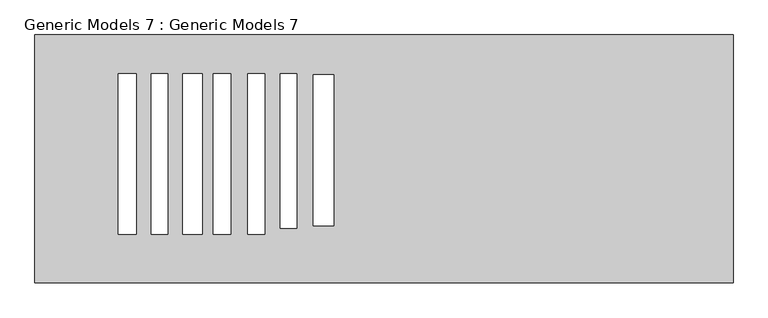
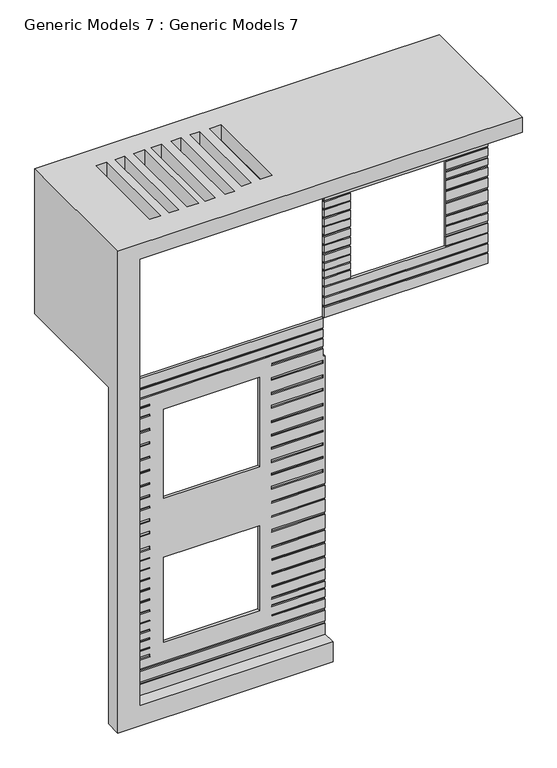
"""IFC4 building model written with IfcOpenShell, lengths in millimetres: proxy geometry, Generic Models 7 : Generic Models 7."""

from ifc_helpers import new_model, si_unit, origin, place, context, project, spatial, faceted_brep, source, transform, mapped, element, save


def generic_models_7_generic_models_7_94141b15(model_context):
    return source(origin(), model_context, "Body", "Brep", [
        faceted_brep([(-19866.491855, -13904.9538163, 3044.3262356), (-19256.891855, -13904.9538163, 3044.3262356), (-19256.891855, -13904.9538163, 3048.6001668), (-17428.091855, -13904.9538163, 3048.6001668), (-17428.091855, -13904.9538163, 3047.830136), (-16170.791855, -13904.9538163, 3047.830136), (-16170.791855, -13904.9538163, 3267.9963637), (-19866.491855, -13904.9538163, 3267.9963637), (-16208.891855, -13904.9538163, 9448.8), (-19866.491855, -13904.9538163, 9448.8), (-19866.491855, -13904.9538163, 9255.7850961), (-16208.891855, -13904.9538163, 9255.7850961), (-16170.791855, -13904.9538163, 8676.8631794), (-16208.891855, -13904.9538163, 8676.8631794), (-16208.891855, -13904.9538163, 8832.7952088), (-17199.491855, -13904.9538163, 8832.7952088), (-17199.491855, -13904.9538163, 8880.0631794), (-16208.891855, -13904.9538163, 8880.0631794), (-16208.891855, -13904.9538163, 9029.746389), (-19866.491855, -13904.9538163, 9029.746389), (-19866.491855, -13904.9538163, 8880.0631794), (-19518.8909009, -13904.9538163, 8880.0631794), (-19518.8909009, -13904.9538163, 8832.7952088), (-19866.491855, -13904.9538163, 8832.7952088), (-19866.491855, -13904.9538163, 8676.8631794), (-19518.8909009, -13904.9538163, 8676.8631794), (-19518.8909009, -13904.9538163, 8634.1909778), (-19866.491855, -13904.9538163, 8634.1909778), (-19866.491855, -13904.9538163, 8392.6341349), (-19518.8909009, -13904.9538163, 8392.6341349), (-19518.8909009, -13904.9538163, 8341.0204513), (-19866.491855, -13904.9538163, 8341.0204513), (-19866.491855, -13904.9538163, 8123.1111078), (-19518.8909009, -13904.9538163, 8123.1111078), (-19518.8909009, -13904.9538163, 8063.5568574), (-19866.491855, -13904.9538163, 8063.5568574), (-19866.491855, -13904.9538163, 7829.3101393), (-19518.8909009, -13904.9538163, 7829.3101393), (-19518.8909009, -13904.9538163, 7789.6073057), (-19866.491855, -13904.9538163, 7789.6073057), (-19866.491855, -13904.9538163, 7560.8382052), (-19518.8909009, -13904.9538163, 7560.8382052), (-19518.8909009, -13904.9538163, 7519.6280374), (-19866.491855, -13904.9538163, 7519.6280374), (-19866.491855, -13904.9538163, 7292.9915007), (-19518.8909009, -13904.9538163, 7292.9915007), (-19518.8909009, -13904.9538163, 7245.6784857), (-19866.491855, -13904.9538163, 7245.6784857), (-19866.491855, -13904.9538163, 7047.1643178), (-19518.8909009, -13904.9538163, 7047.1643178), (-19518.8909009, -13904.9538163, 6995.5506342), (-19866.491855, -13904.9538163, 6995.5506342), (-19866.491855, -13904.9538163, 6812.9175997), (-19518.8909009, -13904.9538163, 6812.9175997), (-19518.8909009, -13904.9538163, 6777.1850495), (-19866.491855, -13904.9538163, 6777.1850495), (-19866.491855, -13904.9538163, 6565.3056423), (-19518.8909009, -13904.9538163, 6565.3056423), (-19518.8909009, -13904.9538163, 6498.8842905), (-19866.491855, -13904.9538163, 6498.8842905), (-19866.491855, -13904.9538163, 6314.0836024), (-19518.8909009, -13904.9538163, 6314.0836024), (-19518.8909009, -13904.9538163, 6245.8245058), (-19866.491855, -13904.9538163, 6245.8245058), (-19866.491855, -13904.9538163, 6004.2923177), (-19518.8909009, -13904.9538163, 6004.2923177), (-19518.8909009, -13904.9538163, 5941.2839209), (-19866.491855, -13904.9538163, 5941.2839209), (-19866.491855, -13904.9538163, 5773.2615291), (-19518.8909009, -13904.9538163, 5773.2615291), (-19518.8909009, -13904.9538163, 5750.6444422), (-19866.491855, -13904.9538163, 5750.6444422), (-19866.491855, -13904.9538163, 5576.5223744), (-19518.8909009, -13904.9538163, 5576.5223744), (-19518.8909009, -13904.9538163, 5549.5034328), (-19866.491855, -13904.9538163, 5549.5034328), (-19866.491855, -13904.9538163, 5375.3813649), (-19518.8909009, -13904.9538163, 5375.3813649), (-19518.8909009, -13904.9538163, 5339.3561095), (-19866.491855, -13904.9538163, 5339.3561095), (-19866.491855, -13904.9538163, 5168.2361463), (-19518.8909009, -13904.9538163, 5168.2361463), (-19518.8909009, -13904.9538163, 5126.2066816), (-19866.491855, -13904.9538163, 5126.2066816), (-19866.491855, -13904.9538163, 4946.0804045), (-19518.8909009, -13904.9538163, 4946.0804045), (-19518.8909009, -13904.9538163, 4904.0509398), (-19866.491855, -13904.9538163, 4904.0509398), (-19866.491855, -13904.9538163, 4723.9246627), (-19518.8909009, -13904.9538163, 4723.9246627), (-19518.8909009, -13904.9538163, 4684.8973027), (-19866.491855, -13904.9538163, 4684.8973027), (-19866.491855, -13904.9538163, 4516.7794441), (-19518.8909009, -13904.9538163, 4516.7794441), (-19518.8909009, -13904.9538163, 4492.7626071), (-19866.491855, -13904.9538163, 4492.7626071), (-19866.491855, -13904.9538163, 4333.6510623), (-19518.8909009, -13904.9538163, 4333.6510623), (-19518.8909009, -13904.9538163, 4291.6215977), (-19866.491855, -13904.9538163, 4291.6215977), (-19866.491855, -13904.9538163, 4156.5855814), (-19518.8909009, -13904.9538163, 4156.5855814), (-19518.8909009, -13904.9538163, 4114.4974252), (-19866.491855, -13904.9538163, 4114.4974252), (-19866.491855, -13904.9538163, 3967.0387154), (-19518.8909009, -13904.9538163, 3967.0387154), (-19518.8909009, -13904.9538163, 3933.6499225), (-19866.491855, -13904.9538163, 3933.6499225), (-19866.491855, -13904.9538163, 3823.2932772), (-19518.8909009, -13904.9538163, 3823.2932772), (-19518.8909009, -13904.9538163, 3767.4448595), (-19866.491855, -13904.9538163, 3767.4448595), (-19866.491855, -13904.9538163, 3581.1876632), (-16170.791855, -13904.9538163, 3581.1876632), (-16170.791855, -13904.9538163, 3767.4448595), (-17199.491855, -13904.9538163, 3767.4448595), (-17199.491855, -13904.9538163, 3803.3089422), (-16170.791855, -13904.9538163, 3803.3089422), (-16170.791855, -13904.9538163, 3967.0387154), (-17199.491855, -13904.9538163, 3967.0387154), (-17199.491855, -13904.9538163, 4001.7088996), (-16170.791855, -13904.9538163, 4001.7088996), (-16170.791855, -13904.9538163, 4116.5720328), (-17199.491855, -13904.9538163, 4116.5720328), (-17199.491855, -13904.9538163, 4156.5855814), (-16170.791855, -13904.9538163, 4156.5855814), (-16170.791855, -13904.9538163, 4346.2982993), (-17199.491855, -13904.9538163, 4346.2982993), (-17199.491855, -13904.9538163, 4382.8456599), (-16170.791855, -13904.9538163, 4382.8456599), (-16170.791855, -13904.9538163, 4605.7845593), (-17199.491855, -13904.9538163, 4605.7845593), (-17199.491855, -13904.9538163, 4647.2829369), (-16170.791855, -13904.9538163, 4647.2829369), (-16170.791855, -13904.9538163, 4888.8830249), (-17199.491855, -13904.9538163, 4888.8830249), (-17199.491855, -13904.9538163, 4930.3120686), (-16170.791855, -13904.9538163, 4930.3120686), (-16170.791855, -13904.9538163, 5147.8145482), (-17199.491855, -13904.9538163, 5147.8145482), (-17199.491855, -13904.9538163, 5189.2435919), (-16170.791855, -13904.9538163, 5189.2435919), (-16170.791855, -13904.9538163, 5472.3420575), (-17199.491855, -13904.9538163, 5472.3420575), (-17199.491855, -13904.9538163, 5524.1283621), (-16170.791855, -13904.9538163, 5524.1283621), (-16170.791855, -13904.9538163, 5772.0121405), (-17199.491855, -13904.9538163, 5772.0121405), (-17199.491855, -13904.9538163, 5806.5363436), (-16170.791855, -13904.9538163, 5806.5363436), (-16170.791855, -13904.9538163, 6055.110606), (-17199.491855, -13904.9538163, 6055.110606), (-17199.491855, -13904.9538163, 6096.0), (-16170.791855, -13904.9538163, 6096.0), (-19256.891855, -13904.9538163, 8676.8631794), (-17428.091855, -13904.9538163, 8676.8631794), (-17428.091855, -13904.9538163, 6875.7032327), (-19256.891855, -13904.9538163, 6875.7032327), (-17428.091855, -13904.9538163, 3967.0387154), (-19256.891855, -13904.9538163, 3967.0387154), (-19256.891855, -13904.9538163, 5684.1406455), (-17428.091855, -13904.9538163, 5684.1406455), (-16208.891855, -13904.9538163, 8591.2496538), (-16208.891855, -13904.9538163, 8537.4008097), (-17199.491855, -13904.9538163, 8537.4008097), (-17199.491855, -13904.9538163, 8591.2496538), (-16208.891855, -13904.9538163, 8299.1838083), (-16208.891855, -13904.9538163, 8247.3975036), (-17199.491855, -13904.9538163, 8247.3975036), (-17199.491855, -13904.9538163, 8299.1838083), (-16208.891855, -13904.9538163, 8029.895024), (-16208.891855, -13904.9538163, 7978.1087193), (-17199.491855, -13904.9538163, 7978.1087193), (-17199.491855, -13904.9538163, 8029.895024), (-16208.891855, -13904.9538163, 7725.553622), (-16208.891855, -13904.9538163, 7677.7481522), (-17199.491855, -13904.9538163, 7677.7481522), (-17199.491855, -13904.9538163, 7725.553622), (-16208.891855, -13904.9538163, 7449.8884117), (-16208.891855, -13904.9538163, 7405.0069477), (-17199.491855, -13904.9538163, 7405.0069477), (-17199.491855, -13904.9538163, 7449.8884117), (-16208.891855, -13904.9538163, 7184.0520477), (-16208.891855, -13904.9538163, 7149.5278446), (-17199.491855, -13904.9538163, 7149.5278446), (-17199.491855, -13904.9538163, 7184.0520477), (-16208.891855, -13904.9538163, 6932.025365), (-16208.891855, -13904.9538163, 6875.7032327), (-17199.491855, -13904.9538163, 6875.7032327), (-17199.491855, -13904.9538163, 6932.025365), (-16208.891855, -13904.9538163, 6655.8317401), (-16208.891855, -13904.9538163, 6617.8551167), (-17199.491855, -13904.9538163, 6617.8551167), (-17199.491855, -13904.9538163, 6655.8317401), (-16208.891855, -13904.9538163, 6393.4477965), (-16208.891855, -13904.9538163, 6338.2090715), (-17199.491855, -13904.9538163, 6338.2090715), (-17199.491855, -13904.9538163, 6393.4477965), (-16208.891855, -13904.9538163, 9062.8315897), (-16208.891855, -13904.9538163, 9218.346183), (-19866.491855, -13904.9538163, 9218.346183), (-19866.491855, -13904.9538163, 9062.8315897), (-16170.791855, -13904.9538163, 3324.930227), (-16170.791855, -13904.9538163, 3536.2157608), (-19866.491855, -13904.9538163, 3536.2157608), (-19866.491855, -13904.9538163, 3324.930227), (-19256.891855, -13854.1538163, 3044.3262356), (-19866.491855, -13854.1538163, 3044.3262356), (-19866.491855, -13854.1538163, 9448.8), (-16208.891855, -13854.1538163, 9448.8), (-16208.891855, -13854.1538163, 8676.8631794), (-16170.791855, -13854.1538163, 8676.8631794), (-16170.791855, -13854.1538163, 3047.830136), (-17428.091855, -13854.1538163, 3047.830136), (-17428.091855, -13854.1538163, 3048.6001668), (-19256.891855, -13854.1538163, 3048.6001668), (-17428.091855, -13854.1538163, 8676.8631794), (-19256.891855, -13854.1538163, 8676.8631794), (-19256.891855, -13854.1538163, 6875.7032327), (-17428.091855, -13854.1538163, 6875.7032327), (-19256.891855, -13854.1538163, 3967.0387154), (-17428.091855, -13854.1538163, 3967.0387154), (-17428.091855, -13854.1538163, 5684.1406455), (-19256.891855, -13854.1538163, 5684.1406455), (-19866.491855, -13879.5538163, 3267.9963637), (-19866.491855, -13879.5538163, 3324.930227), (-19866.491855, -13879.5538163, 3536.2157608), (-19866.491855, -13879.5538163, 3581.1876632), (-19866.491855, -13879.5538163, 3767.4448595), (-19866.491855, -13879.5538163, 3823.2932772), (-19866.491855, -13879.5538163, 3933.6499225), (-19866.491855, -13879.5538163, 3967.0387154), (-19866.491855, -13879.5538163, 4114.4974252), (-19866.491855, -13879.5538163, 4156.5855814), (-19866.491855, -13879.5538163, 4291.6215977), (-19866.491855, -13879.5538163, 4333.6510623), (-19866.491855, -13879.5538163, 4492.7626071), (-19866.491855, -13879.5538163, 4516.7794441), (-19866.491855, -13879.5538163, 4684.8973027), (-19866.491855, -13879.5538163, 4723.9246627), (-19866.491855, -13879.5538163, 4904.0509398), (-19866.491855, -13879.5538163, 4946.0804045), (-19866.491855, -13879.5538163, 5126.2066816), (-19866.491855, -13879.5538163, 5168.2361463), (-19866.491855, -13879.5538163, 5339.3561095), (-19866.491855, -13879.5538163, 5375.3813649), (-19866.491855, -13879.5538163, 5549.5034328), (-19866.491855, -13879.5538163, 5576.5223744), (-19866.491855, -13879.5538163, 5750.6444422), (-19866.491855, -13879.5538163, 5773.2615291), (-19866.491855, -13879.5538163, 5941.2839209), (-19866.491855, -13879.5538163, 6004.2923177), (-19866.491855, -13879.5538163, 6245.8245058), (-19866.491855, -13879.5538163, 6314.0836024), (-19866.491855, -13879.5538163, 6498.8842905), (-19866.491855, -13879.5538163, 6565.3056423), (-19866.491855, -13879.5538163, 6777.1850495), (-19866.491855, -13879.5538163, 6812.9175997), (-19866.491855, -13879.5538163, 6995.5506342), (-19866.491855, -13879.5538163, 7047.1643178), (-19866.491855, -13879.5538163, 7245.6784857), (-19866.491855, -13879.5538163, 7292.9915007), (-19866.491855, -13879.5538163, 7519.6280374), (-19866.491855, -13879.5538163, 7560.8382052), (-19866.491855, -13879.5538163, 7789.6073057), (-19866.491855, -13879.5538163, 7829.3101393), (-19866.491855, -13879.5538163, 8063.5568574), (-19866.491855, -13879.5538163, 8123.1111078), (-19866.491855, -13879.5538163, 8341.0204513), (-19866.491855, -13879.5538163, 8392.6341349), (-19866.491855, -13879.5538163, 8634.1909778), (-19866.491855, -13879.5538163, 8676.8631794), (-19866.491855, -13879.5538163, 8832.7952088), (-19866.491855, -13879.5538163, 8880.0631794), (-19866.491855, -13879.5538163, 9029.746389), (-19866.491855, -13879.5538163, 9062.8315897), (-19866.491855, -13879.5538163, 9218.346183), (-19866.491855, -13879.5538163, 9255.7850961), (-16208.891855, -13879.5538163, 9255.7850961), (-16208.891855, -13879.5538163, 9218.346183), (-16208.891855, -13879.5538163, 9062.8315897), (-16208.891855, -13879.5538163, 9029.746389), (-16208.891855, -13879.5538163, 8880.0631794), (-16208.891855, -13879.5538163, 8832.7952088), (-16170.791855, -13879.5538163, 6096.0), (-16170.791855, -13879.5538163, 6055.110606), (-16170.791855, -13879.5538163, 5806.5363436), (-16170.791855, -13879.5538163, 5772.0121405), (-16170.791855, -13879.5538163, 5524.1283621), (-16170.791855, -13879.5538163, 5472.3420575), (-16170.791855, -13879.5538163, 5189.2435919), (-16170.791855, -13879.5538163, 5147.8145482), (-16170.791855, -13879.5538163, 4930.3120686), (-16170.791855, -13879.5538163, 4888.8830249), (-16170.791855, -13879.5538163, 4647.2829369), (-16170.791855, -13879.5538163, 4605.7845593), (-16170.791855, -13879.5538163, 4382.8456599), (-16170.791855, -13879.5538163, 4346.2982993), (-16170.791855, -13879.5538163, 4156.5855814), (-16170.791855, -13879.5538163, 4116.5720328), (-16170.791855, -13879.5538163, 4001.7088996), (-16170.791855, -13879.5538163, 3967.0387154), (-16170.791855, -13879.5538163, 3803.3089422), (-16170.791855, -13879.5538163, 3767.4448595), (-16170.791855, -13879.5538163, 3581.1876632), (-16170.791855, -13879.5538163, 3536.2157608), (-16170.791855, -13879.5538163, 3324.930227), (-16170.791855, -13879.5538163, 3267.9963637), (-19518.8909009, -13879.5538163, 8832.7952088), (-19518.8909009, -13879.5538163, 8880.0631794), (-19518.8909009, -13879.5538163, 8676.8631794), (-19518.8909009, -13879.5538163, 8634.1909778), (-17199.491855, -13879.5538163, 8880.0631794), (-17199.491855, -13879.5538163, 8832.7952088), (-19518.8909009, -13879.5538163, 8392.6341349), (-19518.8909009, -13879.5538163, 8341.0204513), (-19518.8909009, -13879.5538163, 8123.1111078), (-19518.8909009, -13879.5538163, 8063.5568574), (-19518.8909009, -13879.5538163, 7829.3101393), (-19518.8909009, -13879.5538163, 7789.6073057), (-19518.8909009, -13879.5538163, 7560.8382052), (-19518.8909009, -13879.5538163, 7519.6280374), (-19518.8909009, -13879.5538163, 7292.9915007), (-19518.8909009, -13879.5538163, 7245.6784857), (-19518.8909009, -13879.5538163, 7047.1643178), (-19518.8909009, -13879.5538163, 6995.5506342), (-19518.8909009, -13879.5538163, 6812.9175997), (-19518.8909009, -13879.5538163, 6777.1850495), (-19518.8909009, -13879.5538163, 6565.3056423), (-19518.8909009, -13879.5538163, 6498.8842905), (-19518.8909009, -13879.5538163, 6314.0836024), (-19518.8909009, -13879.5538163, 6245.8245058), (-19518.8909009, -13879.5538163, 6004.2923177), (-19518.8909009, -13879.5538163, 5941.2839209), (-19518.8909009, -13879.5538163, 5773.2615291), (-19518.8909009, -13879.5538163, 5750.6444422), (-19518.8909009, -13879.5538163, 5576.5223744), (-19518.8909009, -13879.5538163, 5549.5034328), (-19518.8909009, -13879.5538163, 5375.3813649), (-19518.8909009, -13879.5538163, 5339.3561095), (-19518.8909009, -13879.5538163, 5168.2361463), (-19518.8909009, -13879.5538163, 5126.2066816), (-19518.8909009, -13879.5538163, 4946.0804045), (-19518.8909009, -13879.5538163, 4904.0509398), (-19518.8909009, -13879.5538163, 4723.9246627), (-19518.8909009, -13879.5538163, 4684.8973027), (-19518.8909009, -13879.5538163, 4516.7794441), (-19518.8909009, -13879.5538163, 4492.7626071), (-19518.8909009, -13879.5538163, 3767.4448595), (-19518.8909009, -13879.5538163, 3823.2932772), (-19518.8909009, -13879.5538163, 4333.6510623), (-19518.8909009, -13879.5538163, 4291.6215977), (-19518.8909009, -13879.5538163, 4156.5855814), (-19518.8909009, -13879.5538163, 4114.4974252), (-19518.8909009, -13879.5538163, 3967.0387154), (-19518.8909009, -13879.5538163, 3933.6499225), (-16208.891855, -13879.5538163, 8591.2496538), (-17199.491855, -13879.5538163, 8591.2496538), (-17199.491855, -13879.5538163, 8537.4008097), (-16208.891855, -13879.5538163, 8537.4008097), (-16208.891855, -13879.5538163, 8299.1838083), (-17199.491855, -13879.5538163, 8299.1838083), (-17199.491855, -13879.5538163, 8247.3975036), (-16208.891855, -13879.5538163, 8247.3975036), (-16208.891855, -13879.5538163, 8029.895024), (-17199.491855, -13879.5538163, 8029.895024), (-17199.491855, -13879.5538163, 7978.1087193), (-16208.891855, -13879.5538163, 7978.1087193), (-16208.891855, -13879.5538163, 7725.553622), (-17199.491855, -13879.5538163, 7725.553622), (-17199.491855, -13879.5538163, 7677.7481522), (-16208.891855, -13879.5538163, 7677.7481522), (-16208.891855, -13879.5538163, 7449.8884117), (-17199.491855, -13879.5538163, 7449.8884117), (-17199.491855, -13879.5538163, 7405.0069477), (-16208.891855, -13879.5538163, 7405.0069477), (-16208.891855, -13879.5538163, 7184.0520477), (-17199.491855, -13879.5538163, 7184.0520477), (-17199.491855, -13879.5538163, 7149.5278446), (-16208.891855, -13879.5538163, 7149.5278446), (-16208.891855, -13879.5538163, 6932.025365), (-17199.491855, -13879.5538163, 6932.025365), (-17199.491855, -13879.5538163, 6875.7032327), (-16208.891855, -13879.5538163, 6875.7032327), (-16208.891855, -13879.5538163, 6655.8317401), (-17199.491855, -13879.5538163, 6655.8317401), (-17199.491855, -13879.5538163, 6617.8551167), (-16208.891855, -13879.5538163, 6617.8551167), (-16208.891855, -13879.5538163, 6393.4477965), (-17199.491855, -13879.5538163, 6393.4477965), (-17199.491855, -13879.5538163, 6338.2090715), (-16208.891855, -13879.5538163, 6338.2090715), (-17199.491855, -13879.5538163, 6096.0), (-17199.491855, -13879.5538163, 6055.110606), (-17199.491855, -13879.5538163, 5806.5363436), (-17199.491855, -13879.5538163, 5772.0121405), (-17199.491855, -13879.5538163, 5524.1283621), (-17199.491855, -13879.5538163, 5472.3420575), (-17199.491855, -13879.5538163, 5189.2435919), (-17199.491855, -13879.5538163, 5147.8145482), (-17199.491855, -13879.5538163, 4930.3120686), (-17199.491855, -13879.5538163, 4888.8830249), (-17199.491855, -13879.5538163, 4647.2829369), (-17199.491855, -13879.5538163, 4605.7845593), (-17199.491855, -13879.5538163, 3803.3089422), (-17199.491855, -13879.5538163, 3767.4448595), (-17199.491855, -13879.5538163, 4382.8456599), (-17199.491855, -13879.5538163, 4346.2982993), (-17199.491855, -13879.5538163, 4156.5855814), (-17199.491855, -13879.5538163, 4116.5720328), (-17199.491855, -13879.5538163, 4001.7088996), (-17199.491855, -13879.5538163, 3967.0387154)], [[[0, 1, 2, 3, 4, 5, 6, 7]], [[8, 9, 10, 11]], [[12, 13, 14, 15, 16, 17, 18, 19, 20, 21, 22, 23, 24, 25, 26, 27, 28, 29, 30, 31, 32, 33, 34, 35, 36, 37, 38, 39, 40, 41, 42, 43, 44, 45, 46, 47, 48, 49, 50, 51, 52, 53, 54, 55, 56, 57, 58, 59, 60, 61, 62, 63, 64, 65, 66, 67, 68, 69, 70, 71, 72, 73, 74, 75, 76, 77, 78, 79, 80, 81, 82, 83, 84, 85, 86, 87, 88, 89, 90, 91, 92, 93, 94, 95, 96, 97, 98, 99, 100, 101, 102, 103, 104, 105, 106, 107, 108, 109, 110, 111, 112, 113, 114, 115, 116, 117, 118, 119, 120, 121, 122, 123, 124, 125, 126, 127, 128, 129, 130, 131, 132, 133, 134, 135, 136, 137, 138, 139, 140, 141, 142, 143, 144, 145, 146, 147, 148, 149, 150, 151, 152, 153], [154, 155, 156, 157], [158, 159, 160, 161], [162, 163, 164, 165], [166, 167, 168, 169], [170, 171, 172, 173], [174, 175, 176, 177], [178, 179, 180, 181], [182, 183, 184, 185], [186, 187, 188, 189], [190, 191, 192, 193], [194, 195, 196, 197]], [[198, 199, 200, 201]], [[202, 203, 204, 205]], [[206, 207, 208, 209, 210, 211, 212, 213, 214, 215], [216, 217, 218, 219], [220, 221, 222, 223]], [[207, 0, 7, 224, 225, 205, 204, 226, 227, 112, 111, 228, 229, 108, 107, 230, 231, 104, 103, 232, 233, 100, 99, 234, 235, 96, 95, 236, 237, 92, 91, 238, 239, 88, 87, 240, 241, 84, 83, 242, 243, 80, 79, 244, 245, 76, 75, 246, 247, 72, 71, 248, 249, 68, 67, 250, 251, 64, 63, 252, 253, 60, 59, 254, 255, 56, 55, 256, 257, 52, 51, 258, 259, 48, 47, 260, 261, 44, 43, 262, 263, 40, 39, 264, 265, 36, 35, 266, 267, 32, 31, 268, 269, 28, 27, 270, 271, 24, 23, 272, 273, 20, 19, 274, 275, 201, 200, 276, 277, 10, 9, 208]], [[1, 0, 207, 206]], [[1, 206, 215, 2]], [[217, 154, 157, 218]], [[159, 220, 223, 160]], [[9, 8, 209, 208]], [[154, 217, 216, 155]], [[210, 209, 8, 11, 278, 279, 199, 198, 280, 281, 18, 17, 282, 283, 14, 13]], [[12, 211, 210, 13]], [[155, 216, 219, 156]], [[213, 4, 3, 214]], [[221, 158, 161, 222]], [[5, 4, 213, 212]], [[212, 211, 12, 153, 284, 285, 150, 149, 286, 287, 146, 145, 288, 289, 142, 141, 290, 291, 138, 137, 292, 293, 134, 133, 294, 295, 130, 129, 296, 297, 126, 125, 298, 299, 122, 121, 300, 301, 118, 117, 302, 303, 114, 113, 304, 305, 203, 202, 306, 307, 6, 5]], [[159, 158, 221, 220]], [[3, 2, 215, 214]], [[157, 156, 219, 218]], [[161, 160, 223, 222]], [[278, 277, 276, 279]], [[280, 275, 274, 281]], [[272, 308, 309, 273]], [[310, 271, 270, 311]], [[282, 312, 313, 283]], [[314, 269, 268, 315]], [[316, 267, 266, 317]], [[318, 265, 264, 319]], [[320, 263, 262, 321]], [[322, 261, 260, 323]], [[324, 259, 258, 325]], [[326, 257, 256, 327]], [[328, 255, 254, 329]], [[330, 253, 252, 331]], [[332, 251, 250, 333]], [[334, 249, 248, 335]], [[336, 247, 246, 337]], [[338, 245, 244, 339]], [[340, 243, 242, 341]], [[342, 241, 240, 343]], [[344, 239, 238, 345]], [[346, 237, 236, 347]], [[228, 348, 349, 229]], [[350, 235, 234, 351]], [[352, 233, 232, 353]], [[354, 231, 230, 355]], [[356, 357, 358, 359]], [[360, 361, 362, 363]], [[364, 365, 366, 367]], [[368, 369, 370, 371]], [[372, 373, 374, 375]], [[376, 377, 378, 379]], [[380, 381, 382, 383]], [[384, 385, 386, 387]], [[388, 389, 390, 391]], [[392, 393, 285, 284]], [[286, 394, 395, 287]], [[288, 396, 397, 289]], [[290, 398, 399, 291]], [[292, 400, 401, 293]], [[402, 403, 295, 294]], [[302, 404, 405, 303]], [[296, 406, 407, 297]], [[298, 408, 409, 299]], [[300, 410, 411, 301]], [[304, 227, 226, 305]], [[306, 225, 224, 307]], [[279, 276, 200, 199]], [[277, 278, 11, 10]], [[281, 274, 19, 18]], [[275, 280, 198, 201]], [[273, 309, 21, 20]], [[309, 308, 22, 21]], [[308, 272, 23, 22]], [[310, 311, 26, 25]], [[311, 270, 27, 26]], [[271, 310, 25, 24]], [[283, 313, 15, 14]], [[313, 312, 16, 15]], [[312, 282, 17, 16]], [[314, 315, 30, 29]], [[315, 268, 31, 30]], [[269, 314, 29, 28]], [[316, 317, 34, 33]], [[317, 266, 35, 34]], [[267, 316, 33, 32]], [[318, 319, 38, 37]], [[319, 264, 39, 38]], [[265, 318, 37, 36]], [[320, 321, 42, 41]], [[321, 262, 43, 42]], [[263, 320, 41, 40]], [[322, 323, 46, 45]], [[323, 260, 47, 46]], [[261, 322, 45, 44]], [[324, 325, 50, 49]], [[325, 258, 51, 50]], [[259, 324, 49, 48]], [[326, 327, 54, 53]], [[327, 256, 55, 54]], [[257, 326, 53, 52]], [[328, 329, 58, 57]], [[329, 254, 59, 58]], [[255, 328, 57, 56]], [[330, 331, 62, 61]], [[331, 252, 63, 62]], [[253, 330, 61, 60]], [[332, 333, 66, 65]], [[333, 250, 67, 66]], [[251, 332, 65, 64]], [[334, 335, 70, 69]], [[335, 248, 71, 70]], [[249, 334, 69, 68]], [[336, 337, 74, 73]], [[337, 246, 75, 74]], [[247, 336, 73, 72]], [[338, 339, 78, 77]], [[339, 244, 79, 78]], [[245, 338, 77, 76]], [[340, 341, 82, 81]], [[341, 242, 83, 82]], [[243, 340, 81, 80]], [[342, 343, 86, 85]], [[343, 240, 87, 86]], [[241, 342, 85, 84]], [[344, 345, 90, 89]], [[345, 238, 91, 90]], [[239, 344, 89, 88]], [[346, 347, 94, 93]], [[347, 236, 95, 94]], [[237, 346, 93, 92]], [[229, 349, 109, 108]], [[349, 348, 110, 109]], [[348, 228, 111, 110]], [[350, 351, 98, 97]], [[351, 234, 99, 98]], [[235, 350, 97, 96]], [[352, 353, 102, 101]], [[353, 232, 103, 102]], [[233, 352, 101, 100]], [[354, 355, 106, 105]], [[355, 230, 107, 106]], [[231, 354, 105, 104]], [[356, 359, 163, 162]], [[359, 358, 164, 163]], [[358, 357, 165, 164]], [[357, 356, 162, 165]], [[360, 363, 167, 166]], [[363, 362, 168, 167]], [[362, 361, 169, 168]], [[361, 360, 166, 169]], [[364, 367, 171, 170]], [[367, 366, 172, 171]], [[366, 365, 173, 172]], [[365, 364, 170, 173]], [[368, 371, 175, 174]], [[371, 370, 176, 175]], [[370, 369, 177, 176]], [[369, 368, 174, 177]], [[372, 375, 179, 178]], [[375, 374, 180, 179]], [[374, 373, 181, 180]], [[373, 372, 178, 181]], [[376, 379, 183, 182]], [[379, 378, 184, 183]], [[378, 377, 185, 184]], [[377, 376, 182, 185]], [[380, 383, 187, 186]], [[383, 382, 188, 187]], [[382, 381, 189, 188]], [[381, 380, 186, 189]], [[384, 387, 191, 190]], [[387, 386, 192, 191]], [[386, 385, 193, 192]], [[385, 384, 190, 193]], [[388, 391, 195, 194]], [[391, 390, 196, 195]], [[390, 389, 197, 196]], [[389, 388, 194, 197]], [[392, 284, 153, 152]], [[285, 393, 151, 150]], [[393, 392, 152, 151]], [[287, 395, 147, 146]], [[395, 394, 148, 147]], [[394, 286, 149, 148]], [[289, 397, 143, 142]], [[397, 396, 144, 143]], [[396, 288, 145, 144]], [[291, 399, 139, 138]], [[399, 398, 140, 139]], [[398, 290, 141, 140]], [[293, 401, 135, 134]], [[401, 400, 136, 135]], [[400, 292, 137, 136]], [[402, 294, 133, 132]], [[295, 403, 131, 130]], [[403, 402, 132, 131]], [[303, 405, 115, 114]], [[405, 404, 116, 115]], [[404, 302, 117, 116]], [[297, 407, 127, 126]], [[407, 406, 128, 127]], [[406, 296, 129, 128]], [[299, 409, 123, 122]], [[409, 408, 124, 123]], [[408, 298, 125, 124]], [[301, 411, 119, 118]], [[411, 410, 120, 119]], [[410, 300, 121, 120]], [[305, 226, 204, 203]], [[227, 304, 113, 112]], [[307, 224, 7, 6]], [[225, 306, 202, 205]]]),
        faceted_brep([(-13059.291855, -13904.9538163, 12073.6764103), (-16196.191855, -13904.9538163, 12073.6764103), (-16196.191855, -13904.9538163, 11963.7380132), (-13059.291855, -13904.9538163, 11963.7380132), (-16196.191855, -13904.9538163, 9448.8), (-13059.291855, -13904.9538163, 9448.8), (-13059.291855, -13904.9538163, 9654.3858981), (-16196.191855, -13904.9538163, 9654.3858981), (-13859.391855, -13904.9538163, 11785.0777387), (-13859.391855, -13904.9538163, 11620.9674566), (-13059.291855, -13904.9538163, 11620.9674566), (-13059.291855, -13904.9538163, 11785.0777387), (-13859.391855, -13904.9538163, 11573.5445728), (-13859.391855, -13904.9538163, 11443.4517052), (-13059.291855, -13904.9538163, 11443.4517052), (-13059.291855, -13904.9538163, 11573.5445728), (-13859.391855, -13904.9538163, 11395.7873478), (-13859.391855, -13904.9538163, 11222.3244377), (-13059.291855, -13904.9538163, 11222.3244377), (-13059.291855, -13904.9538163, 11395.7873478), (-13859.391855, -13904.9538163, 11177.4429737), (-13859.391855, -13904.9538163, 10984.1074362), (-13059.291855, -13904.9538163, 10984.1074362), (-13059.291855, -13904.9538163, 11177.4429737), (-13859.391855, -13904.9538163, 10938.1106834), (-13859.391855, -13904.9538163, 10717.7255453), (-13059.291855, -13904.9538163, 10717.7255453), (-13059.291855, -13904.9538163, 10938.1106834), (-13859.391855, -13904.9538163, 10668.0), (-13859.391855, -13904.9538163, 10497.9780712), (-13059.291855, -13904.9538163, 10497.9780712), (-13059.291855, -13904.9538163, 10668.0), (-13859.391855, -13904.9538163, 10257.7104416), (-13859.391855, -13904.9538163, 10082.0304475), (-13059.291855, -13904.9538163, 10082.0304475), (-13059.291855, -13904.9538163, 10257.7104416), (-13859.391855, -13904.9538163, 10466.2443896), (-13859.391855, -13904.9538163, 10307.4330552), (-13059.291855, -13904.9538163, 10307.4330552), (-13059.291855, -13904.9538163, 10466.2443896), (-15688.191855, -13904.9538163, 11649.6832399), (-15688.191855, -13904.9538163, 11785.0777387), (-16196.191855, -13904.9538163, 11785.0777387), (-16196.191855, -13904.9538163, 11649.6832399), (-15688.191855, -13904.9538163, 11477.3885401), (-15688.191855, -13904.9538163, 11620.9674566), (-16196.191855, -13904.9538163, 11620.9674566), (-16196.191855, -13904.9538163, 11477.3885401), (-15688.191855, -13904.9538163, 11297.2622629), (-15688.191855, -13904.9538163, 11443.4517052), (-16196.191855, -13904.9538163, 11443.4517052), (-16196.191855, -13904.9538163, 11297.2622629), (-15688.191855, -13904.9538163, 11117.1359858), (-15688.191855, -13904.9538163, 11273.7675311), (-16196.191855, -13904.9538163, 11273.7675311), (-16196.191855, -13904.9538163, 11117.1359858), (-15688.191855, -13904.9538163, 10926.5676057), (-15688.191855, -13904.9538163, 11080.5886253), (-16196.191855, -13904.9538163, 11080.5886253), (-16196.191855, -13904.9538163, 10926.5676057), (-15688.191855, -13904.9538163, 10761.2382052), (-15688.191855, -13904.9538163, 10900.4623482), (-16196.191855, -13904.9538163, 10900.4623482), (-16196.191855, -13904.9538163, 10761.2382052), (-15688.191855, -13904.9538163, 10566.3150515), (-15688.191855, -13904.9538163, 10717.7255453), (-16196.191855, -13904.9538163, 10717.7255453), (-16196.191855, -13904.9538163, 10566.3150515), (-15688.191855, -13904.9538163, 10413.6511106), (-15688.191855, -13904.9538163, 10542.8203197), (-16196.191855, -13904.9538163, 10542.8203197), (-16196.191855, -13904.9538163, 10413.6511106), (-15688.191855, -13904.9538163, 10082.0304475), (-15688.191855, -13904.9538163, 10230.0753864), (-16196.191855, -13904.9538163, 10230.0753864), (-16196.191855, -13904.9538163, 10082.0304475), (-15688.191855, -13904.9538163, 10257.7104416), (-15688.191855, -13904.9538163, 10387.9899878), (-16196.191855, -13904.9538163, 10387.9899878), (-16196.191855, -13904.9538163, 10257.7104416), (-13059.291855, -13904.9538163, 9688.7653872), (-13059.291855, -13904.9538163, 9846.5205936), (-16196.191855, -13904.9538163, 9846.5205936), (-16196.191855, -13904.9538163, 9688.7653872), (-16196.191855, -13904.9538163, 11818.3759079), (-13059.291855, -13904.9538163, 11818.3759079), (-13059.291855, -13904.9538163, 11937.1367557), (-16196.191855, -13904.9538163, 11937.1367557), (-13059.291855, -13904.9538163, 10057.845459), (-16196.191855, -13904.9538163, 10057.845459), (-16196.191855, -13904.9538163, 9876.5416398), (-13059.291855, -13904.9538163, 9876.5416398), (-16196.191855, -13854.1538163, 12073.6764103), (-13059.291855, -13854.1538163, 12073.6764103), (-13059.291855, -13854.1538163, 9448.8), (-16196.191855, -13854.1538163, 9448.8), (-13859.391855, -13854.1538163, 11818.3759079), (-15688.191855, -13854.1538163, 11818.3759079), (-15688.191855, -13854.1538163, 10057.845459), (-13859.391855, -13854.1538163, 10057.845459), (-16196.191855, -13879.5538163, 9654.3858981), (-16196.191855, -13879.5538163, 9688.7653872), (-16196.191855, -13879.5538163, 9846.5205936), (-16196.191855, -13879.5538163, 9876.5416398), (-16196.191855, -13879.5538163, 10057.845459), (-16196.191855, -13879.5538163, 10082.0304475), (-16196.191855, -13879.5538163, 10230.0753864), (-16196.191855, -13879.5538163, 10257.7104416), (-16196.191855, -13879.5538163, 10387.9899878), (-16196.191855, -13879.5538163, 10413.6511106), (-16196.191855, -13879.5538163, 10542.8203197), (-16196.191855, -13879.5538163, 10566.3150515), (-16196.191855, -13879.5538163, 10717.7255453), (-16196.191855, -13879.5538163, 10761.2382052), (-16196.191855, -13879.5538163, 10900.4623482), (-16196.191855, -13879.5538163, 10926.5676057), (-16196.191855, -13879.5538163, 11080.5886253), (-16196.191855, -13879.5538163, 11117.1359858), (-16196.191855, -13879.5538163, 11273.7675311), (-16196.191855, -13879.5538163, 11297.2622629), (-16196.191855, -13879.5538163, 11443.4517052), (-16196.191855, -13879.5538163, 11477.3885401), (-16196.191855, -13879.5538163, 11620.9674566), (-16196.191855, -13879.5538163, 11649.6832399), (-16196.191855, -13879.5538163, 11785.0777387), (-16196.191855, -13879.5538163, 11818.3759079), (-16196.191855, -13879.5538163, 11937.1367557), (-16196.191855, -13879.5538163, 11963.7380132), (-15688.191855, -13879.5538163, 11818.3759079), (-15688.191855, -13879.5538163, 11785.0777387), (-15688.191855, -13879.5538163, 11649.6832399), (-15688.191855, -13879.5538163, 11620.9674566), (-15688.191855, -13879.5538163, 11477.3885401), (-15688.191855, -13879.5538163, 11443.4517052), (-15688.191855, -13879.5538163, 11297.2622629), (-15688.191855, -13879.5538163, 11273.7675311), (-15688.191855, -13879.5538163, 11117.1359858), (-15688.191855, -13879.5538163, 11080.5886253), (-15688.191855, -13879.5538163, 10926.5676057), (-15688.191855, -13879.5538163, 10900.4623482), (-15688.191855, -13879.5538163, 10761.2382052), (-15688.191855, -13879.5538163, 10717.7255453), (-15688.191855, -13879.5538163, 10566.3150515), (-15688.191855, -13879.5538163, 10542.8203197), (-15688.191855, -13879.5538163, 10413.6511106), (-15688.191855, -13879.5538163, 10387.9899878), (-15688.191855, -13879.5538163, 10257.7104416), (-15688.191855, -13879.5538163, 10230.0753864), (-15688.191855, -13879.5538163, 10082.0304475), (-15688.191855, -13879.5538163, 10057.845459), (-13859.391855, -13879.5538163, 11818.3759079), (-13059.291855, -13879.5538163, 11818.3759079), (-13059.291855, -13879.5538163, 11963.7380132), (-13059.291855, -13879.5538163, 11937.1367557), (-13059.291855, -13879.5538163, 11785.0777387), (-13059.291855, -13879.5538163, 11620.9674566), (-13059.291855, -13879.5538163, 11573.5445728), (-13059.291855, -13879.5538163, 11443.4517052), (-13059.291855, -13879.5538163, 11395.7873478), (-13059.291855, -13879.5538163, 11222.3244377), (-13059.291855, -13879.5538163, 11177.4429737), (-13059.291855, -13879.5538163, 10984.1074362), (-13059.291855, -13879.5538163, 10938.1106834), (-13059.291855, -13879.5538163, 10717.7255453), (-13059.291855, -13879.5538163, 10668.0), (-13059.291855, -13879.5538163, 10497.9780712), (-13059.291855, -13879.5538163, 10466.2443896), (-13059.291855, -13879.5538163, 10307.4330552), (-13059.291855, -13879.5538163, 10257.7104416), (-13059.291855, -13879.5538163, 10082.0304475), (-13059.291855, -13879.5538163, 10057.845459), (-13059.291855, -13879.5538163, 9876.5416398), (-13059.291855, -13879.5538163, 9846.5205936), (-13059.291855, -13879.5538163, 9688.7653872), (-13059.291855, -13879.5538163, 9654.3858981), (-13859.391855, -13879.5538163, 10057.845459), (-13859.391855, -13879.5538163, 10082.0304475), (-13859.391855, -13879.5538163, 10257.7104416), (-13859.391855, -13879.5538163, 10307.4330552), (-13859.391855, -13879.5538163, 10466.2443896), (-13859.391855, -13879.5538163, 10497.9780712), (-13859.391855, -13879.5538163, 10668.0), (-13859.391855, -13879.5538163, 10717.7255453), (-13859.391855, -13879.5538163, 10938.1106834), (-13859.391855, -13879.5538163, 10984.1074362), (-13859.391855, -13879.5538163, 11177.4429737), (-13859.391855, -13879.5538163, 11222.3244377), (-13859.391855, -13879.5538163, 11395.7873478), (-13859.391855, -13879.5538163, 11443.4517052), (-13859.391855, -13879.5538163, 11573.5445728), (-13859.391855, -13879.5538163, 11620.9674566), (-13859.391855, -13879.5538163, 11785.0777387)], [[[0, 1, 2, 3]], [[4, 5, 6, 7]], [[8, 9, 10, 11]], [[12, 13, 14, 15]], [[16, 17, 18, 19]], [[20, 21, 22, 23]], [[24, 25, 26, 27]], [[28, 29, 30, 31]], [[32, 33, 34, 35]], [[36, 37, 38, 39]], [[40, 41, 42, 43]], [[44, 45, 46, 47]], [[48, 49, 50, 51]], [[52, 53, 54, 55]], [[56, 57, 58, 59]], [[60, 61, 62, 63]], [[64, 65, 66, 67]], [[68, 69, 70, 71]], [[72, 73, 74, 75]], [[76, 77, 78, 79]], [[80, 81, 82, 83]], [[84, 85, 86, 87]], [[88, 89, 90, 91]], [[92, 93, 94, 95], [96, 97, 98, 99]], [[95, 4, 7, 100, 101, 83, 82, 102, 103, 90, 89, 104, 105, 75, 74, 106, 107, 79, 78, 108, 109, 71, 70, 110, 111, 67, 66, 112, 113, 63, 62, 114, 115, 59, 58, 116, 117, 55, 54, 118, 119, 51, 50, 120, 121, 47, 46, 122, 123, 43, 42, 124, 125, 84, 87, 126, 127, 2, 1, 92]], [[4, 95, 94, 5]], [[98, 97, 128, 129, 41, 40, 130, 131, 45, 44, 132, 133, 49, 48, 134, 135, 53, 52, 136, 137, 57, 56, 138, 139, 61, 60, 140, 141, 65, 64, 142, 143, 69, 68, 144, 145, 77, 76, 146, 147, 73, 72, 148, 149]], [[1, 0, 93, 92]], [[84, 125, 128, 97, 96, 150, 151, 85]], [[93, 0, 3, 152, 153, 86, 85, 151, 154, 11, 10, 155, 156, 15, 14, 157, 158, 19, 18, 159, 160, 23, 22, 161, 162, 27, 26, 163, 164, 31, 30, 165, 166, 39, 38, 167, 168, 35, 34, 169, 170, 88, 91, 171, 172, 81, 80, 173, 174, 6, 5, 94]], [[96, 99, 175, 176, 33, 32, 177, 178, 37, 36, 179, 180, 29, 28, 181, 182, 25, 24, 183, 184, 21, 20, 185, 186, 17, 16, 187, 188, 13, 12, 189, 190, 9, 8, 191, 150]], [[88, 170, 175, 99, 98, 149, 104, 89]], [[151, 150, 191, 154]], [[104, 149, 148, 105]], [[152, 127, 126, 153]], [[124, 129, 128, 125]], [[130, 123, 122, 131]], [[132, 121, 120, 133]], [[134, 119, 118, 135]], [[136, 117, 116, 137]], [[138, 115, 114, 139]], [[140, 113, 112, 141]], [[142, 111, 110, 143]], [[144, 109, 108, 145]], [[146, 107, 106, 147]], [[155, 190, 189, 156]], [[157, 188, 187, 158]], [[159, 186, 185, 160]], [[161, 184, 183, 162]], [[163, 182, 181, 164]], [[169, 176, 175, 170]], [[165, 180, 179, 166]], [[167, 178, 177, 168]], [[171, 103, 102, 172]], [[173, 101, 100, 174]], [[153, 126, 87, 86]], [[127, 152, 3, 2]], [[154, 191, 8, 11]], [[129, 124, 42, 41]], [[131, 122, 46, 45]], [[123, 130, 40, 43]], [[133, 120, 50, 49]], [[121, 132, 44, 47]], [[135, 118, 54, 53]], [[119, 134, 48, 51]], [[137, 116, 58, 57]], [[117, 136, 52, 55]], [[139, 114, 62, 61]], [[115, 138, 56, 59]], [[141, 112, 66, 65]], [[113, 140, 60, 63]], [[143, 110, 70, 69]], [[111, 142, 64, 67]], [[105, 148, 72, 75]], [[145, 108, 78, 77]], [[109, 144, 68, 71]], [[147, 106, 74, 73]], [[107, 146, 76, 79]], [[156, 189, 12, 15]], [[190, 155, 10, 9]], [[158, 187, 16, 19]], [[188, 157, 14, 13]], [[160, 185, 20, 23]], [[186, 159, 18, 17]], [[162, 183, 24, 27]], [[184, 161, 22, 21]], [[164, 181, 28, 31]], [[182, 163, 26, 25]], [[176, 169, 34, 33]], [[166, 179, 36, 39]], [[180, 165, 30, 29]], [[168, 177, 32, 35]], [[178, 167, 38, 37]], [[172, 102, 82, 81]], [[103, 171, 91, 90]], [[174, 100, 7, 6]], [[101, 173, 80, 83]]]),
        faceted_brep([(-19866.491855, -14158.9538163, 3048.0), (-19866.491855, -14158.9538163, 12073.6764103), (-12551.291855, -14158.9538163, 12073.6764103), (-12551.291855, -14158.9538163, 12378.4764103), (-20285.591855, -14158.9538163, 12378.4764103), (-20285.591855, -14158.9538163, 2645.3232141), (-16170.791855, -14158.9538163, 2645.3232141), (-16170.791855, -14158.9538163, 3048.0), (-16170.791855, -13854.1538163, 3048.0), (-16170.791855, -13854.1538163, 2645.3232141), (-20285.591855, -13854.1538163, 2645.3232141), (-20285.591855, -13854.1538163, 9448.8), (-19866.491855, -13854.1538163, 9448.8), (-19866.491855, -13854.1538163, 3048.0), (-19866.491855, -11415.7538163, 9448.8), (-19866.491855, -11415.7538163, 12073.6764103), (-20285.591855, -11415.7538163, 12378.4764103), (-20285.591855, -11415.7538163, 9448.8), (-12551.291855, -11415.7538163, 12378.4764103), (-12551.291855, -11415.7538163, 12073.6764103), (-19160.8773376, -13625.5538163, 12378.4764103), (-19364.0773376, -13625.5538163, 12378.4764103), (-19364.0773376, -11847.5538163, 12378.4764103), (-19160.8773376, -11847.5538163, 12378.4764103), (-18816.1892204, -13625.5538163, 12378.4764103), (-18998.7690322, -13625.5538163, 12378.4764103), (-18998.7690322, -11847.5538163, 12378.4764103), (-18816.1892204, -11847.5538163, 12378.4764103), (-18431.4936356, -13625.5538163, 12378.4764103), (-18647.9749064, -13625.5538163, 12378.4764103), (-18647.9749064, -11847.5538163, 12378.4764103), (-18431.4936356, -11847.5538163, 12378.4764103), (-18114.0828733, -13625.5538163, 12378.4764103), (-18309.8913874, -13625.5538163, 12378.4764103), (-18309.8913874, -11847.5538163, 12378.4764103), (-18114.0828733, -11847.5538163, 12378.4764103), (-17740.0450362, -13625.5538163, 12378.4764103), (-17925.1958026, -13625.5538163, 12378.4764103), (-17925.1958026, -11847.5538163, 12378.4764103), (-17740.0450362, -11847.5538163, 12378.4764103), (-17382.6988808, -13554.8994663, 12378.4764103), (-17567.791855, -13554.8994663, 12378.4764103), (-17567.791855, -11847.5538163, 12378.4764103), (-17382.6988808, -11847.5538163, 12378.4764103), (-16974.2477038, -13531.2154888, 12378.4764103), (-17202.8477038, -13531.2154888, 12378.4764103), (-17202.8477038, -11854.8154888, 12378.4764103), (-16974.2477038, -11854.8154888, 12378.4764103), (-19364.0773376, -13625.5538163, 12073.6764103), (-19160.8773376, -13625.5538163, 12073.6764103), (-19160.8773376, -11847.5538163, 12073.6764103), (-19364.0773376, -11847.5538163, 12073.6764103), (-18998.7690322, -13625.5538163, 12073.6764103), (-18816.1892204, -13625.5538163, 12073.6764103), (-18816.1892204, -11847.5538163, 12073.6764103), (-18998.7690322, -11847.5538163, 12073.6764103), (-18647.9749064, -13625.5538163, 12073.6764103), (-18431.4936356, -13625.5538163, 12073.6764103), (-18431.4936356, -11847.5538163, 12073.6764103), (-18647.9749064, -11847.5538163, 12073.6764103), (-18309.8913874, -13625.5538163, 12073.6764103), (-18114.0828733, -13625.5538163, 12073.6764103), (-18114.0828733, -11847.5538163, 12073.6764103), (-18309.8913874, -11847.5538163, 12073.6764103), (-17925.1958026, -13625.5538163, 12073.6764103), (-17740.0450362, -13625.5538163, 12073.6764103), (-17740.0450362, -11847.5538163, 12073.6764103), (-17925.1958026, -11847.5538163, 12073.6764103), (-17567.791855, -13554.8994663, 12073.6764103), (-17382.6988808, -13554.8994663, 12073.6764103), (-17382.6988808, -11847.5538163, 12073.6764103), (-17567.791855, -11847.5538163, 12073.6764103), (-17202.8477038, -13531.2154888, 12073.6764103), (-16974.2477038, -13531.2154888, 12073.6764103), (-16974.2477038, -11854.8154888, 12073.6764103), (-17202.8477038, -11854.8154888, 12073.6764103)], [[[0, 1, 2, 3, 4, 5, 6, 7]], [[8, 9, 10, 11, 12, 13]], [[1, 0, 13, 12, 14, 15]], [[10, 5, 4, 16, 17, 11]], [[6, 5, 10, 9]], [[7, 6, 9, 8]], [[7, 8, 13, 0]], [[11, 17, 14, 12]], [[14, 17, 16, 18, 19, 15]], [[3, 18, 16, 4], [20, 21, 22, 23], [24, 25, 26, 27], [28, 29, 30, 31], [32, 33, 34, 35], [36, 37, 38, 39], [40, 41, 42, 43], [44, 45, 46, 47]], [[19, 2, 1, 15], [48, 49, 50, 51], [52, 53, 54, 55], [56, 57, 58, 59], [60, 61, 62, 63], [64, 65, 66, 67], [68, 69, 70, 71], [72, 73, 74, 75]], [[18, 3, 2, 19]], [[48, 21, 20, 49]], [[21, 48, 51, 22]], [[22, 51, 50, 23]], [[49, 20, 23, 50]], [[52, 25, 24, 53]], [[25, 52, 55, 26]], [[26, 55, 54, 27]], [[53, 24, 27, 54]], [[56, 29, 28, 57]], [[29, 56, 59, 30]], [[30, 59, 58, 31]], [[57, 28, 31, 58]], [[60, 33, 32, 61]], [[33, 60, 63, 34]], [[34, 63, 62, 35]], [[61, 32, 35, 62]], [[64, 37, 36, 65]], [[37, 64, 67, 38]], [[38, 67, 66, 39]], [[65, 36, 39, 66]], [[68, 41, 40, 69]], [[41, 68, 71, 42]], [[42, 71, 70, 43]], [[69, 40, 43, 70]], [[72, 45, 44, 73]], [[45, 72, 75, 46]], [[46, 75, 74, 47]], [[73, 44, 47, 74]]]),
    ])


if __name__ == "__main__":
    model = new_model("IFC4")
    model_context = context("Model", 3, world=origin())
    ifc_project = project(units=[si_unit("LENGTHUNIT", "METRE", prefix="MILLI")], contexts=[model_context])
    site = spatial("IfcSite", under=ifc_project)
    building = spatial("IfcBuilding", under=site)
    placement = place(None, origin())
    generic_models_7_generic_models_7_shape = generic_models_7_generic_models_7_94141b15(model_context)
    element("IfcBuildingElementProxy", 1, Name="Generic Models 7 : Generic Models 7", ObjectType="Generic Models 7 : Generic Models 7", at=placement, inside=building, context=model_context, shape_type="MappedRepresentation", body=[
        mapped(generic_models_7_generic_models_7_shape, transform((0.0, 0.0, 0.0), x_axis=(1.0, 0.0, 0.0), y_axis=(0.0, 1.0, 0.0), z_axis=(0.0, 0.0, 1.0))),
    ])
    save(model, "model.ifc")
